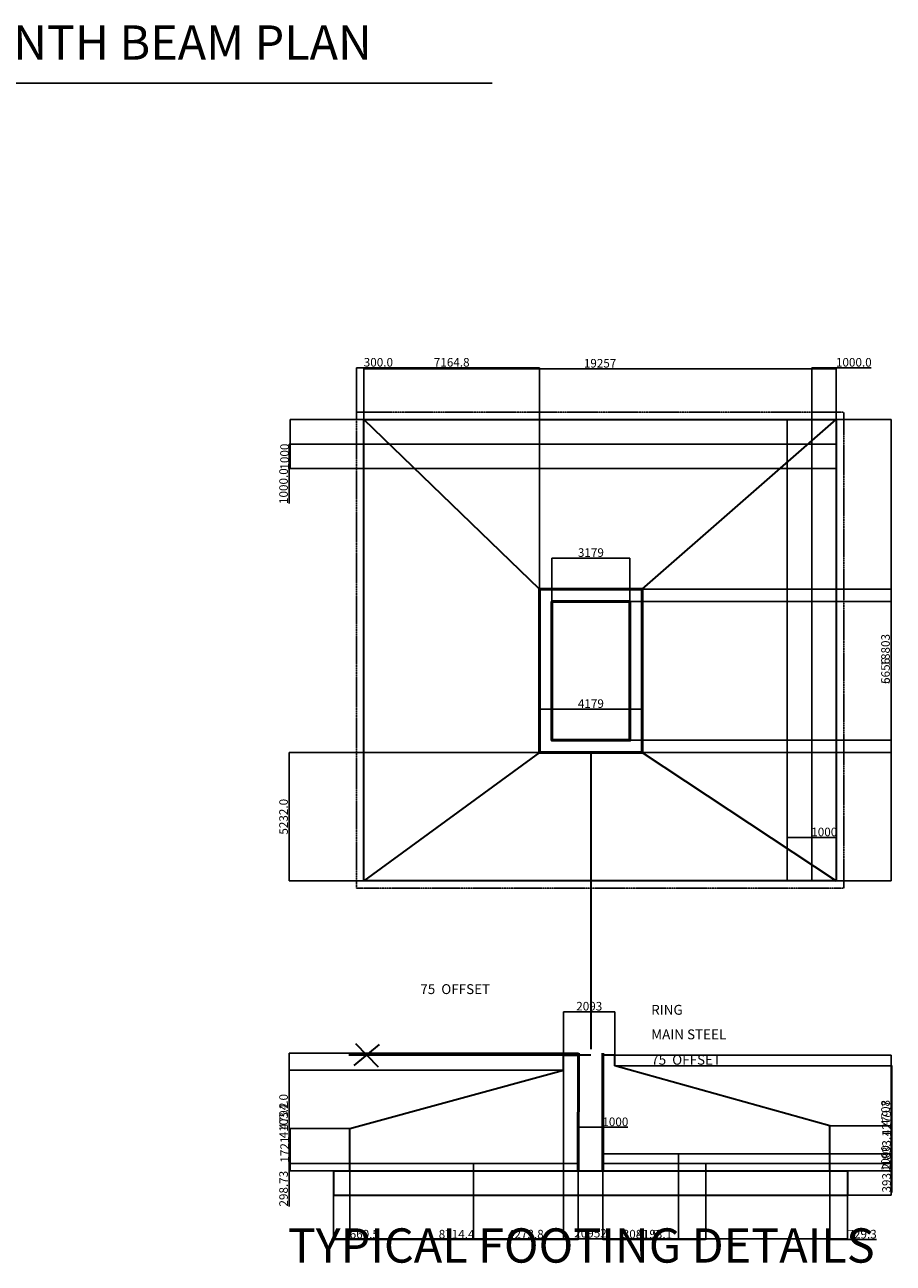
# Model space of a CAD drawing. Units: millimetres. Extents: x -2405 to 73447, y 417 to 55353.
# Tile 3 of 3: x 38054 to 73447, y 4879 to 55353. Entities that reach past the tile are written whole.
import ezdxf

# ---------------------------------------------------------------- set-up
doc = ezdxf.new("R2010")
doc.units = ezdxf.units.MM
doc.linetypes.add('DASHED', pattern=[19.05, 12.7, -6.35])
for name, color, linetype, lineweight in [('S-ANNO-DIMS', 2, 'Continuous', 18), ('S-ANNO-TEXT', 7, 'Continuous', 25), ('S-COLS', 4, 'Continuous', 50), ('S-FNDN', 3, 'Continuous', 35), ('S-FNDN-HIDN', 8, 'DASHED', 25), ('S-REIN', 1, 'Continuous', 25)]:
    doc.layers.add(name, color=color, linetype=linetype, lineweight=lineweight)
doc.styles.get("Standard").update_dxf_attribs({"font": 'arial.ttf'})
doc.dimstyles.new('ISO-25', dxfattribs={"dimtxt": 350, "dimasz": 2.5, "dimexe": 1.25, "dimexo": 0.625, "dimtad": 1, "dimdec": 0, "dimtxsty": 'Standard', "dimcen": 2.5, "dimadec": 0, "dimazin": 0, "dimtfac": 1, "dimtdec": 0, "dimtmove": 0, "dimatfit": 3, "dimfxl": 1, "dimarcsym": 0})

# ---------------------------------------------------------------- blocks, each defined once
blk = doc.blocks.new('*D23')
at = {"layer": 'Defpoints', "color": 0, "transparency": 16777216}
for p in [(71128, 41333), (51872, 39263), (71128, 39263)]:
    blk.add_point(p, dxfattribs=at)
at = {"layer": 'S-ANNO-DIMS', "color": 0, "lineweight": -2, "transparency": 16777216}
for p, q in [((51872, 39263), (51872, 41334)), ((51874, 41333), (71126, 41333)), ((71128, 39263), (71128, 41334))]:
    blk.add_line(p, q, dxfattribs=at)
at = {"layer": 'S-ANNO-DIMS', "color": 0, "transparency": 16777216}
for points in [[(51874, 41333), (51874, 41332), (51872, 41333)], [(71126, 41333), (71126, 41332), (71128, 41333)]]:
    blk.add_solid(points, dxfattribs=at)
at = {"layer": 'S-ANNO-DIMS', "color": 0, "transparency": 16777216, "insert": (61500, 41512), "char_height": 350, "attachment_point": 5}
blk.add_mtext('19257', dxfattribs=at)
blk = doc.blocks.new('*D24')
at = {"layer": 'Defpoints', "color": 0, "transparency": 16777216}
for p in [(71128, 39263), (71128, 20460), (73357, 20460)]:
    blk.add_point(p, dxfattribs=at)
at = {"layer": 'S-ANNO-DIMS', "color": 0, "lineweight": -2, "transparency": 16777216}
for p, q in [((71129, 39263), (73358, 39263)), ((73357, 39260), (73357, 20463)), ((71129, 20460), (73358, 20460))]:
    blk.add_line(p, q, dxfattribs=at)
at = {"layer": 'S-ANNO-DIMS', "color": 0, "transparency": 16777216}
for points in [[(73357, 39260), (73358, 39260), (73357, 39263)], [(73357, 20463), (73358, 20463), (73357, 20460)]]:
    blk.add_solid(points, dxfattribs=at)
at = {"layer": 'S-ANNO-DIMS', "color": 0, "transparency": 16777216, "insert": (73178, 29862), "char_height": 350, "attachment_point": 5, "rotation": 90}
blk.add_mtext('18803', dxfattribs=at)
blk = doc.blocks.new('*D25')
at = {"layer": 'Defpoints', "color": 0, "transparency": 16777216}
for p in [(63215, 27462), (59036, 25692), (63215, 25692)]:
    blk.add_point(p, dxfattribs=at)
at = {"layer": 'S-ANNO-DIMS', "color": 0, "lineweight": -2, "transparency": 16777216}
for p, q in [((59036, 25693), (59036, 27464)), ((59039, 27462), (63213, 27462)), ((63215, 25693), (63215, 27464))]:
    blk.add_line(p, q, dxfattribs=at)
at = {"layer": 'S-ANNO-DIMS', "color": 0, "transparency": 16777216}
for points in [[(59039, 27463), (59039, 27462), (59036, 27462)], [(63213, 27463), (63213, 27462), (63215, 27462)]]:
    blk.add_solid(points, dxfattribs=at)
at = {"layer": 'S-ANNO-DIMS', "color": 0, "transparency": 16777216, "insert": (61126, 27642), "char_height": 350, "attachment_point": 5}
blk.add_mtext('4179', dxfattribs=at)
blk = doc.blocks.new('*D26')
at = {"layer": 'Defpoints', "color": 0, "transparency": 16777216}
for p in [(63215, 32348), (63215, 25692), (73357, 25692)]:
    blk.add_point(p, dxfattribs=at)
at = {"layer": 'S-ANNO-DIMS', "color": 0, "lineweight": -2, "transparency": 16777216}
for p, q in [((63216, 32348), (73358, 32348)), ((73357, 32346), (73357, 25695)), ((63216, 25692), (73358, 25692))]:
    blk.add_line(p, q, dxfattribs=at)
at = {"layer": 'S-ANNO-DIMS', "color": 0, "transparency": 16777216}
for points in [[(73357, 32346), (73358, 32346), (73357, 32348)], [(73357, 25695), (73358, 25695), (73357, 25692)]]:
    blk.add_solid(points, dxfattribs=at)
at = {"layer": 'S-ANNO-DIMS', "color": 0, "transparency": 16777216, "insert": (73178, 29020), "char_height": 350, "attachment_point": 5, "rotation": 90}
blk.add_mtext('6656', dxfattribs=at)
blk = doc.blocks.new('*D27')
at = {"layer": 'Defpoints', "color": 0, "transparency": 16777216}
for p in [(62715, 33618), (59536, 31848), (62715, 31848)]:
    blk.add_point(p, dxfattribs=at)
at = {"layer": 'S-ANNO-DIMS', "color": 0, "lineweight": -2, "transparency": 16777216}
for p, q in [((59536, 31849), (59536, 33619)), ((59539, 33618), (62713, 33618)), ((62715, 31849), (62715, 33619))]:
    blk.add_line(p, q, dxfattribs=at)
at = {"layer": 'S-ANNO-DIMS', "color": 0, "transparency": 16777216}
for points in [[(59539, 33618), (59539, 33618), (59536, 33618)], [(62713, 33618), (62713, 33618), (62715, 33618)]]:
    blk.add_solid(points, dxfattribs=at)
at = {"layer": 'S-ANNO-DIMS', "color": 0, "transparency": 16777216, "insert": (61126, 33797), "char_height": 350, "attachment_point": 5}
blk.add_mtext('3179', dxfattribs=at)
blk = doc.blocks.new('*D28')
at = {"layer": 'Defpoints', "color": 0, "transparency": 16777216}
for p in [(62715, 31848), (62715, 26192), (73357, 26192)]:
    blk.add_point(p, dxfattribs=at)
at = {"layer": 'S-ANNO-DIMS', "color": 0, "lineweight": -2, "transparency": 16777216}
for p, q in [((62716, 31848), (73358, 31848)), ((73357, 31846), (73357, 26195)), ((62716, 26192), (73358, 26192))]:
    blk.add_line(p, q, dxfattribs=at)
at = {"layer": 'S-ANNO-DIMS', "color": 0, "transparency": 16777216}
for points in [[(73357, 31846), (73358, 31846), (73357, 31848)], [(73357, 26195), (73358, 26195), (73357, 26192)]]:
    blk.add_solid(points, dxfattribs=at)
at = {"layer": 'S-ANNO-DIMS', "color": 0, "transparency": 16777216, "insert": (73178, 29020), "char_height": 350, "attachment_point": 5, "rotation": 90}
blk.add_mtext('5656', dxfattribs=at)
blk = doc.blocks.new('*D29')
at = {"layer": 'Defpoints', "color": 0, "transparency": 16777216}
for p in [(70128, 22230), (69128, 20460), (70128, 20460)]:
    blk.add_point(p, dxfattribs=at)
at = {"layer": 'S-ANNO-DIMS', "color": 0, "lineweight": -2, "transparency": 16777216}
for p, q in [((69128, 20461), (69128, 22232)), ((69131, 22230), (70126, 22230)), ((70128, 20461), (70128, 22232)), ((70128, 22230), (71143, 22230))]:
    blk.add_line(p, q, dxfattribs=at)
at = {"layer": 'S-ANNO-DIMS', "color": 0, "transparency": 16777216}
for points in [[(69131, 22231), (69131, 22230), (69128, 22230)], [(70126, 22231), (70126, 22230), (70128, 22230)]]:
    blk.add_solid(points, dxfattribs=at)
at = {"layer": 'S-ANNO-DIMS', "color": 0, "transparency": 16777216, "insert": (70637, 22410), "char_height": 350, "attachment_point": 5}
blk.add_mtext('1000', dxfattribs=at)
blk = doc.blocks.new('*D30')
at = {"layer": 'Defpoints', "color": 0, "transparency": 16777216}
for p in [(51872, 39263), (48866, 38263), (51872, 38263)]:
    blk.add_point(p, dxfattribs=at)
at = {"layer": 'S-ANNO-DIMS', "color": 0, "lineweight": -2, "transparency": 16777216}
for p, q in [((51871, 39263), (48864, 39263)), ((48866, 39260), (48866, 38265)), ((51871, 38263), (48864, 38263)), ((48866, 38263), (48866, 37248))]:
    blk.add_line(p, q, dxfattribs=at)
at = {"layer": 'S-ANNO-DIMS', "color": 0, "transparency": 16777216}
for points in [[(48865, 39260), (48866, 39260), (48866, 39263)], [(48865, 38265), (48866, 38265), (48866, 38263)]]:
    blk.add_solid(points, dxfattribs=at)
at = {"layer": 'S-ANNO-DIMS', "color": 0, "transparency": 16777216, "insert": (48686, 37754), "char_height": 350, "attachment_point": 5, "rotation": 90}
blk.add_mtext('1000', dxfattribs=at)
blk = doc.blocks.new('*D31')
at = {"layer": 'Defpoints', "color": 0, "transparency": 16777216}
for p in [(50636, 7650), (71587, 7650), (71587, 5880)]:
    blk.add_point(p, dxfattribs=at)
at = {"layer": 'S-ANNO-DIMS', "color": 0, "lineweight": -2, "transparency": 16777216}
for p, q in [((50636, 7650), (50636, 5879)), ((71587, 7650), (71587, 5879)), ((50638, 5880), (71585, 5880))]:
    blk.add_line(p, q, dxfattribs=at)
at = {"layer": 'S-ANNO-DIMS', "color": 0, "transparency": 16777216}
for points in [[(50638, 5881), (50638, 5880), (50636, 5880)], [(71585, 5881), (71585, 5880), (71587, 5880)]]:
    blk.add_solid(points, dxfattribs=at)
at = {"layer": 'S-ANNO-DIMS', "color": 0, "transparency": 16777216, "insert": (61111, 6059), "char_height": 350, "attachment_point": 5}
blk.add_mtext('20952', dxfattribs=at)
blk = doc.blocks.new('*D32')
at = {"layer": 'Defpoints', "color": 0, "transparency": 16777216}
for p in [(71587, 8650), (73357, 8650), (71587, 7650)]:
    blk.add_point(p, dxfattribs=at)
at = {"layer": 'S-ANNO-DIMS', "color": 0, "lineweight": -2, "transparency": 16777216}
for p, q in [((73357, 8650), (73357, 9665)), ((71588, 8650), (73358, 8650)), ((73357, 7653), (73357, 8648)), ((71588, 7650), (73358, 7650))]:
    blk.add_line(p, q, dxfattribs=at)
at = {"layer": 'S-ANNO-DIMS', "color": 0, "transparency": 16777216}
for points in [[(73357, 8648), (73358, 8648), (73357, 8650)], [(73357, 7653), (73358, 7653), (73357, 7650)]]:
    blk.add_solid(points, dxfattribs=at)
at = {"layer": 'S-ANNO-DIMS', "color": 0, "transparency": 16777216, "insert": (73178, 9159), "char_height": 350, "attachment_point": 5, "rotation": 90}
blk.add_mtext('1000', dxfattribs=at)
blk = doc.blocks.new('*D33')
at = {"layer": 'Defpoints', "color": 0, "transparency": 16777216}
for p in [(48866, 10371), (51296, 10371), (51296, 8650)]:
    blk.add_point(p, dxfattribs=at)
at = {"layer": 'S-ANNO-DIMS', "color": 0, "lineweight": -2, "transparency": 16777216}
for p, q in [((51295, 10371), (48864, 10371)), ((48866, 8653), (48866, 10369)), ((51295, 8650), (48864, 8650))]:
    blk.add_line(p, q, dxfattribs=at)
at = {"layer": 'S-ANNO-DIMS', "color": 0, "transparency": 16777216}
for points in [[(48865, 10369), (48866, 10369), (48866, 10371)], [(48865, 8653), (48866, 8653), (48866, 8650)]]:
    blk.add_solid(points, dxfattribs=at)
at = {"layer": 'S-ANNO-DIMS', "color": 0, "transparency": 16777216, "insert": (48689, 9511), "char_height": 350, "attachment_point": 5, "rotation": 90}
blk.add_mtext('1721', dxfattribs=at)
blk = doc.blocks.new('*D34')
at = {"layer": 'Defpoints', "color": 0, "transparency": 16777216}
for p in [(62103, 13359), (70858, 8650), (73357, 8650)]:
    blk.add_point(p, dxfattribs=at)
at = {"layer": 'S-ANNO-DIMS', "color": 0, "lineweight": -2, "transparency": 16777216}
for p, q in [((62104, 13359), (73358, 13359)), ((73357, 13356), (73357, 8653)), ((70858, 8650), (73358, 8650))]:
    blk.add_line(p, q, dxfattribs=at)
at = {"layer": 'S-ANNO-DIMS', "color": 0, "transparency": 16777216}
for points in [[(73357, 13356), (73358, 13356), (73357, 13359)], [(73357, 8653), (73358, 8653), (73357, 8650)]]:
    blk.add_solid(points, dxfattribs=at)
at = {"layer": 'S-ANNO-DIMS', "color": 0, "transparency": 16777216, "insert": (73178, 11004), "char_height": 350, "attachment_point": 5, "rotation": 90}
blk.add_mtext('4708', dxfattribs=at)
blk = doc.blocks.new('*D35')
at = {"layer": 'Defpoints', "color": 0, "transparency": 16777216}
for p in [(62105, 15129), (60011, 13361), (62103, 13359)]:
    blk.add_point(p, dxfattribs=at)
at = {"layer": 'S-ANNO-DIMS', "color": 0, "lineweight": -2, "transparency": 16777216}
for p, q in [((60011, 13361), (60012, 15132)), ((60015, 15131), (62103, 15129)), ((62103, 13359), (62105, 15130))]:
    blk.add_line(p, q, dxfattribs=at)
at = {"layer": 'S-ANNO-DIMS', "color": 0, "transparency": 16777216}
for points in [[(60015, 15131), (60015, 15130), (60012, 15131)], [(62103, 15129), (62103, 15128), (62105, 15129)]]:
    blk.add_solid(points, dxfattribs=at)
at = {"layer": 'S-ANNO-DIMS', "color": 0, "transparency": 16777216, "insert": (61059, 15309), "char_height": 350, "attachment_point": 5, "rotation": 359.9376}
blk.add_mtext('2093', dxfattribs=at)
blk = doc.blocks.new('*D36')
at = {"layer": 'Defpoints', "color": 0, "transparency": 16777216}
for p in [(61613, 10420), (60611, 8651), (61611, 8650)]:
    blk.add_point(p, dxfattribs=at)
at = {"layer": 'S-ANNO-DIMS', "color": 0, "lineweight": -2, "transparency": 16777216}
for p, q in [((60611, 8651), (60613, 10422)), ((60616, 10421), (61611, 10420)), ((61611, 8650), (61613, 10421)), ((61613, 10420), (62628, 10418))]:
    blk.add_line(p, q, dxfattribs=at)
at = {"layer": 'S-ANNO-DIMS', "color": 0, "transparency": 16777216}
for points in [[(60616, 10421), (60616, 10420), (60613, 10421)], [(61611, 10420), (61611, 10419), (61613, 10420)]]:
    blk.add_solid(points, dxfattribs=at)
at = {"layer": 'S-ANNO-DIMS', "color": 0, "transparency": 16777216, "insert": (62122, 10598), "char_height": 350, "attachment_point": 5, "rotation": 359.9376}
blk.add_mtext('1000', dxfattribs=at)
blk = doc.blocks.new('*D46')
at = {"layer": 'Defpoints', "color": 0, "transparency": 16777216}
for p in [(59036, 41373), (51872, 39263), (59036, 32348)]:
    blk.add_point(p, dxfattribs=at)
at = {"layer": 'S-ANNO-DIMS', "color": 0, "lineweight": -2, "transparency": 16777216}
for p, q in [((51872, 39263), (51872, 41374)), ((51874, 41373), (59034, 41373)), ((59036, 32349), (59036, 41374))]:
    blk.add_line(p, q, dxfattribs=at)
at = {"layer": 'S-ANNO-DIMS', "color": 0, "transparency": 16777216}
for points in [[(51874, 41373), (51874, 41372), (51872, 41373)], [(59034, 41373), (59034, 41372), (59036, 41373)]]:
    blk.add_solid(points, dxfattribs=at)
at = {"layer": 'S-ANNO-DIMS', "color": 0, "transparency": 16777216, "insert": (55454, 41552), "char_height": 350, "attachment_point": 5}
blk.add_mtext('7164.8', dxfattribs=at)
blk = doc.blocks.new('*D47')
at = {"layer": 'Defpoints', "color": 0, "transparency": 16777216}
for p in [(59036, 25692), (48826, 20460), (51872, 20460)]:
    blk.add_point(p, dxfattribs=at)
at = {"layer": 'S-ANNO-DIMS', "color": 0, "lineweight": -2, "transparency": 16777216}
for p, q in [((59036, 25692), (48824, 25692)), ((48826, 25690), (48826, 20463)), ((51871, 20460), (48824, 20460))]:
    blk.add_line(p, q, dxfattribs=at)
at = {"layer": 'S-ANNO-DIMS', "color": 0, "transparency": 16777216}
for points in [[(48825, 25690), (48826, 25690), (48826, 25692)], [(48825, 20463), (48826, 20463), (48826, 20460)]]:
    blk.add_solid(points, dxfattribs=at)
at = {"layer": 'S-ANNO-DIMS', "color": 0, "transparency": 16777216, "insert": (48646, 23076), "char_height": 350, "attachment_point": 5, "rotation": 90}
blk.add_mtext('5232.0', dxfattribs=at)
blk = doc.blocks.new('*D48')
at = {"layer": 'Defpoints', "color": 0, "transparency": 16777216}
for p in [(51872, 38263), (48826, 37263), (51872, 37263)]:
    blk.add_point(p, dxfattribs=at)
at = {"layer": 'S-ANNO-DIMS', "color": 0, "lineweight": -2, "transparency": 16777216}
for p, q in [((51871, 38263), (48824, 38263)), ((48826, 38260), (48826, 37265)), ((51871, 37263), (48824, 37263)), ((48826, 37263), (48826, 35840))]:
    blk.add_line(p, q, dxfattribs=at)
at = {"layer": 'S-ANNO-DIMS', "color": 0, "transparency": 16777216}
for points in [[(48825, 38260), (48826, 38260), (48826, 38263)], [(48825, 37265), (48826, 37265), (48826, 37263)]]:
    blk.add_solid(points, dxfattribs=at)
at = {"layer": 'S-ANNO-DIMS', "color": 0, "transparency": 16777216, "insert": (48646, 36550), "char_height": 350, "attachment_point": 5, "rotation": 90}
blk.add_mtext('1000.0', dxfattribs=at)
blk = doc.blocks.new('*D49')
at = {"layer": 'Defpoints', "color": 0, "transparency": 16777216}
for p in [(71128, 41373), (70128, 39263), (71128, 39263)]:
    blk.add_point(p, dxfattribs=at)
at = {"layer": 'S-ANNO-DIMS', "color": 0, "lineweight": -2, "transparency": 16777216}
for p, q in [((70128, 39263), (70128, 41374)), ((70131, 41373), (71126, 41373)), ((71128, 39263), (71128, 41374)), ((71128, 41373), (72551, 41373))]:
    blk.add_line(p, q, dxfattribs=at)
at = {"layer": 'S-ANNO-DIMS', "color": 0, "transparency": 16777216}
for points in [[(70131, 41373), (70131, 41372), (70128, 41373)], [(71126, 41373), (71126, 41372), (71128, 41373)]]:
    blk.add_solid(points, dxfattribs=at)
at = {"layer": 'S-ANNO-DIMS', "color": 0, "transparency": 16777216, "insert": (71841, 41552), "char_height": 350, "attachment_point": 5}
blk.add_mtext('1000.0', dxfattribs=at)
blk = doc.blocks.new('*D50')
at = {"layer": 'Defpoints', "color": 0, "transparency": 16777216}
for p in [(51872, 41373), (51572, 39563), (51872, 39263)]:
    blk.add_point(p, dxfattribs=at)
at = {"layer": 'S-ANNO-DIMS', "color": 0, "lineweight": -2, "transparency": 16777216}
for p, q in [((51572, 39563), (51572, 41374)), ((51574, 41373), (51869, 41373)), ((51872, 39263), (51872, 41374)), ((51872, 41373), (53055, 41373))]:
    blk.add_line(p, q, dxfattribs=at)
at = {"layer": 'S-ANNO-DIMS', "color": 0, "transparency": 16777216}
for points in [[(51574, 41373), (51574, 41372), (51572, 41373)], [(51869, 41373), (51869, 41372), (51872, 41373)]]:
    blk.add_solid(points, dxfattribs=at)
at = {"layer": 'S-ANNO-DIMS', "color": 0, "transparency": 16777216, "insert": (52465, 41552), "char_height": 350, "attachment_point": 5}
blk.add_mtext('300.0', dxfattribs=at)
blk = doc.blocks.new('*D51')
at = {"layer": 'Defpoints', "color": 0, "transparency": 16777216}
for p in [(50636, 8650), (51296, 8650), (51296, 5840)]:
    blk.add_point(p, dxfattribs=at)
at = {"layer": 'S-ANNO-DIMS', "color": 0, "lineweight": -2, "transparency": 16777216}
for p, q in [((50636, 8650), (50636, 5839)), ((51296, 8650), (51296, 5839)), ((50638, 5840), (51294, 5840)), ((51296, 5840), (52485, 5840))]:
    blk.add_line(p, q, dxfattribs=at)
at = {"layer": 'S-ANNO-DIMS', "color": 0, "transparency": 16777216}
for points in [[(50638, 5841), (50638, 5840), (50636, 5840)], [(51294, 5841), (51294, 5840), (51296, 5840)]]:
    blk.add_solid(points, dxfattribs=at)
at = {"layer": 'S-ANNO-DIMS', "color": 0, "transparency": 16777216, "insert": (51892, 6019), "char_height": 350, "attachment_point": 5}
blk.add_mtext('660.5', dxfattribs=at)
blk = doc.blocks.new('*D52')
at = {"layer": 'Defpoints', "color": 0, "transparency": 16777216}
for p in [(70858, 8650), (71587, 8650), (71587, 5840)]:
    blk.add_point(p, dxfattribs=at)
at = {"layer": 'S-ANNO-DIMS', "color": 0, "lineweight": -2, "transparency": 16777216}
for p, q in [((70858, 8650), (70858, 5839)), ((71587, 8650), (71587, 5839)), ((70860, 5840), (71585, 5840)), ((71587, 5840), (72769, 5840))]:
    blk.add_line(p, q, dxfattribs=at)
at = {"layer": 'S-ANNO-DIMS', "color": 0, "transparency": 16777216}
for points in [[(70860, 5841), (70860, 5840), (70858, 5840)], [(71585, 5841), (71585, 5840), (71587, 5840)]]:
    blk.add_solid(points, dxfattribs=at)
at = {"layer": 'S-ANNO-DIMS', "color": 0, "transparency": 16777216, "insert": (72179, 6020), "char_height": 350, "attachment_point": 5}
blk.add_mtext('729.3', dxfattribs=at)
blk = doc.blocks.new('*D53')
at = {"layer": 'Defpoints', "color": 0, "transparency": 16777216}
for p in [(70858, 10483), (70858, 8650), (73397, 8650)]:
    blk.add_point(p, dxfattribs=at)
at = {"layer": 'S-ANNO-DIMS', "color": 0, "lineweight": -2, "transparency": 16777216}
for p, q in [((70858, 10483), (73398, 10483)), ((73397, 10481), (73397, 8653)), ((70858, 8650), (73398, 8650))]:
    blk.add_line(p, q, dxfattribs=at)
at = {"layer": 'S-ANNO-DIMS', "color": 0, "transparency": 16777216}
for points in [[(73397, 10481), (73398, 10481), (73397, 10483)], [(73397, 8653), (73398, 8653), (73397, 8650)]]:
    blk.add_solid(points, dxfattribs=at)
at = {"layer": 'S-ANNO-DIMS', "color": 0, "transparency": 16777216, "insert": (73218, 9567), "char_height": 350, "attachment_point": 5, "rotation": 90}
blk.add_mtext('1833.1', dxfattribs=at)
blk = doc.blocks.new('*D54')
at = {"layer": 'Defpoints', "color": 0, "transparency": 16777216}
for p in [(60011, 12754), (48826, 8651), (60611, 8651)]:
    blk.add_point(p, dxfattribs=at)
at = {"layer": 'S-ANNO-DIMS', "color": 0, "lineweight": -2, "transparency": 16777216}
for p, q in [((60010, 12754), (48824, 12754)), ((48826, 12751), (48826, 8653)), ((60611, 8651), (48824, 8651))]:
    blk.add_line(p, q, dxfattribs=at)
at = {"layer": 'S-ANNO-DIMS', "color": 0, "transparency": 16777216}
for points in [[(48825, 12751), (48826, 12751), (48826, 12754)], [(48825, 8653), (48826, 8653), (48826, 8651)]]:
    blk.add_solid(points, dxfattribs=at)
at = {"layer": 'S-ANNO-DIMS', "color": 0, "transparency": 16777216, "insert": (48646, 10702), "char_height": 350, "attachment_point": 5, "rotation": 90}
blk.add_mtext('4103.2', dxfattribs=at)
blk = doc.blocks.new('*D55')
at = {"layer": 'Defpoints', "color": 0, "transparency": 16777216}
for p in [(60011, 12754), (51296, 10371), (60011, 5840)]:
    blk.add_point(p, dxfattribs=at)
at = {"layer": 'S-ANNO-DIMS', "color": 0, "lineweight": -2, "transparency": 16777216}
for p, q in [((60011, 12753), (60011, 5839)), ((51296, 10370), (51296, 5839)), ((51299, 5840), (60008, 5840))]:
    blk.add_line(p, q, dxfattribs=at)
at = {"layer": 'S-ANNO-DIMS', "color": 0, "transparency": 16777216}
for points in [[(51299, 5841), (51299, 5840), (51296, 5840)], [(60008, 5841), (60008, 5840), (60011, 5840)]]:
    blk.add_solid(points, dxfattribs=at)
at = {"layer": 'S-ANNO-DIMS', "color": 0, "transparency": 16777216, "insert": (55653, 6019), "char_height": 350, "attachment_point": 5}
blk.add_mtext('8714.4', dxfattribs=at)
blk = doc.blocks.new('*D56')
at = {"layer": 'Defpoints', "color": 0, "transparency": 16777216}
for p in [(62103, 12929), (61611, 8650), (73397, 8650)]:
    blk.add_point(p, dxfattribs=at)
at = {"layer": 'S-ANNO-DIMS', "color": 0, "lineweight": -2, "transparency": 16777216}
for p, q in [((62104, 12929), (73398, 12929)), ((73397, 12927), (73397, 8652)), ((61612, 8650), (73398, 8650))]:
    blk.add_line(p, q, dxfattribs=at)
at = {"layer": 'S-ANNO-DIMS', "color": 0, "transparency": 16777216}
for points in [[(73397, 12927), (73398, 12927), (73397, 12929)], [(73397, 8652), (73398, 8652), (73397, 8650)]]:
    blk.add_solid(points, dxfattribs=at)
at = {"layer": 'S-ANNO-DIMS', "color": 0, "transparency": 16777216, "insert": (73218, 10789), "char_height": 350, "attachment_point": 5, "rotation": 90}
blk.add_mtext('4279.7', dxfattribs=at)
blk = doc.blocks.new('*D57')
at = {"layer": 'Defpoints', "color": 0, "transparency": 16777216}
for p in [(56338, 8949), (60612, 8949), (60612, 5840)]:
    blk.add_point(p, dxfattribs=at)
at = {"layer": 'S-ANNO-DIMS', "color": 0, "lineweight": -2, "transparency": 16777216}
for p, q in [((56338, 8948), (56338, 5839)), ((60612, 8948), (60612, 5839)), ((56340, 5840), (60609, 5840))]:
    blk.add_line(p, q, dxfattribs=at)
at = {"layer": 'S-ANNO-DIMS', "color": 0, "transparency": 16777216}
for points in [[(56340, 5841), (56340, 5840), (56338, 5840)], [(60609, 5841), (60609, 5840), (60612, 5840)]]:
    blk.add_solid(points, dxfattribs=at)
at = {"layer": 'S-ANNO-DIMS', "color": 0, "transparency": 16777216, "insert": (58475, 6020), "char_height": 350, "attachment_point": 5}
blk.add_mtext('4273.8', dxfattribs=at)
blk = doc.blocks.new('*D58')
at = {"layer": 'Defpoints', "color": 0, "transparency": 16777216}
for p in [(48826, 8650), (56338, 8949), (56338, 8650)]:
    blk.add_point(p, dxfattribs=at)
at = {"layer": 'S-ANNO-DIMS', "color": 0, "lineweight": -2, "transparency": 16777216}
for p, q in [((56337, 8949), (48824, 8949)), ((56337, 8650), (48824, 8650)), ((48826, 8946), (48826, 8653)), ((48826, 8650), (48826, 7187))]:
    blk.add_line(p, q, dxfattribs=at)
at = {"layer": 'S-ANNO-DIMS', "color": 0, "transparency": 16777216}
for points in [[(48825, 8946), (48826, 8946), (48826, 8949)], [(48825, 8653), (48826, 8653), (48826, 8650)]]:
    blk.add_solid(points, dxfattribs=at)
at = {"layer": 'S-ANNO-DIMS', "color": 0, "transparency": 16777216, "insert": (48646, 7918), "char_height": 350, "attachment_point": 5, "rotation": 90}
blk.add_mtext('298.73', dxfattribs=at)
blk = doc.blocks.new('*D59')
at = {"layer": 'Defpoints', "color": 0, "transparency": 16777216}
for p in [(61612, 8949), (65805, 8949), (65805, 5840)]:
    blk.add_point(p, dxfattribs=at)
at = {"layer": 'S-ANNO-DIMS', "color": 0, "lineweight": -2, "transparency": 16777216}
for p, q in [((61612, 8948), (61612, 5839)), ((65805, 8948), (65805, 5839)), ((61614, 5840), (65802, 5840))]:
    blk.add_line(p, q, dxfattribs=at)
at = {"layer": 'S-ANNO-DIMS', "color": 0, "transparency": 16777216}
for points in [[(61614, 5841), (61614, 5840), (61612, 5840)], [(65802, 5841), (65802, 5840), (65805, 5840)]]:
    blk.add_solid(points, dxfattribs=at)
at = {"layer": 'S-ANNO-DIMS', "color": 0, "transparency": 16777216, "insert": (63708, 6020), "char_height": 350, "attachment_point": 5}
blk.add_mtext('4193.1', dxfattribs=at)
blk = doc.blocks.new('*D60')
at = {"layer": 'Defpoints', "color": 0, "transparency": 16777216}
for p in [(61612, 9342), (64694, 9342), (64694, 5840)]:
    blk.add_point(p, dxfattribs=at)
at = {"layer": 'S-ANNO-DIMS', "color": 0, "lineweight": -2, "transparency": 16777216}
for p, q in [((61612, 9341), (61612, 5839)), ((64694, 9341), (64694, 5839)), ((61615, 5840), (64691, 5840))]:
    blk.add_line(p, q, dxfattribs=at)
at = {"layer": 'S-ANNO-DIMS', "color": 0, "transparency": 16777216}
for points in [[(61615, 5841), (61615, 5840), (61612, 5840)], [(64691, 5841), (64691, 5840), (64694, 5840)]]:
    blk.add_solid(points, dxfattribs=at)
at = {"layer": 'S-ANNO-DIMS', "color": 0, "transparency": 16777216, "insert": (63153, 6020), "char_height": 350, "attachment_point": 5}
blk.add_mtext('3081.5', dxfattribs=at)
blk = doc.blocks.new('*D61')
at = {"layer": 'Defpoints', "color": 0, "transparency": 16777216}
for p in [(64694, 9342), (64694, 8949), (73397, 8949)]:
    blk.add_point(p, dxfattribs=at)
at = {"layer": 'S-ANNO-DIMS', "color": 0, "lineweight": -2, "transparency": 16777216}
for p, q in [((64694, 9342), (73398, 9342)), ((73397, 9340), (73397, 8951)), ((64694, 8949), (73398, 8949)), ((73397, 8949), (73397, 7768))]:
    blk.add_line(p, q, dxfattribs=at)
at = {"layer": 'S-ANNO-DIMS', "color": 0, "transparency": 16777216}
for points in [[(73397, 9340), (73398, 9340), (73397, 9342)], [(73397, 8951), (73398, 8951), (73397, 8949)]]:
    blk.add_solid(points, dxfattribs=at)
at = {"layer": 'S-ANNO-DIMS', "color": 0, "transparency": 16777216, "insert": (73218, 8357), "char_height": 350, "attachment_point": 5, "rotation": 90}
blk.add_mtext('393.2', dxfattribs=at)
blk = doc.blocks.new('*D62')
at = {"layer": 'Defpoints', "color": 0, "transparency": 16777216}
for p in [(60617, 13445), (48826, 8651), (60611, 8651)]:
    blk.add_point(p, dxfattribs=at)
at = {"layer": 'S-ANNO-DIMS', "color": 0, "lineweight": -2, "transparency": 16777216}
for p, q in [((60616, 13445), (48824, 13445)), ((48826, 13442), (48826, 8653)), ((60611, 8651), (48824, 8651))]:
    blk.add_line(p, q, dxfattribs=at)
at = {"layer": 'S-ANNO-DIMS', "color": 0, "transparency": 16777216}
for points in [[(48825, 13442), (48826, 13442), (48826, 13445)], [(48825, 8653), (48826, 8653), (48826, 8651)]]:
    blk.add_solid(points, dxfattribs=at)
at = {"layer": 'S-ANNO-DIMS', "color": 0, "transparency": 16777216, "insert": (48646, 11048), "char_height": 350, "attachment_point": 5, "rotation": 90}
blk.add_mtext('4794.0', dxfattribs=at)

msp = doc.modelspace()

# ---------------------------------------------------------------- linework, layer by layer
at = {"layer": 'S-ANNO-TEXT'}
msp.add_line((-2404.637, 52969.195), (57098.008, 52969.195), dxfattribs=at)
at = {"layer": 'S-COLS'}
for p, q in [((60616.568, 13444.714), (60611.346, 8650.682)), ((61616.567, 13443.625), (61611.346, 8649.593))]:
    msp.add_line(p, q, dxfattribs=at)
for points in [[(59036.384, 32348.004), (63215.45, 32348.004), (63215.45, 25692.289), (59036.384, 25692.289)], [(59536.384, 31848.004), (62715.45, 31848.004), (62715.45, 26192.289), (59536.384, 26192.289)]]:
    msp.add_lwpolyline(points, close=True, dxfattribs=at)
at = {"layer": 'S-FNDN'}
for p, q in [((51871.574, 39262.806), (71128.374, 39262.806)), ((51871.574, 20460.3), (51871.574, 39262.806)), ((59036.384, 32348.004), (51871.574, 39262.806)), ((63215.45, 32348.004), (71128.374, 39262.806)), ((71128.374, 39262.806), (71128.374, 20460.3)), ((59036.384, 25692.289), (51871.574, 20460.3)), ((61125.917, 25692.289), (61125.917, 13608.951)), ((63215.45, 25692.289), (71128.374, 20460.3)), ((71128.374, 20460.3), (51871.574, 20460.3)), ((51479.692, 12939.469), (52507.49, 13796.926)), ((51528.059, 13839.195), (52459.123, 12879.085)), ((61125.917, 13359.612), (51264.684, 13359.612)), ((60010.529, 13360.827), (60616.476, 13360.167)), ((60010.529, 12753.871), (60010.529, 13360.827)), ((62103.494, 13358.547), (61616.475, 13359.078)), ((62103.494, 12929.297), (62103.494, 13358.547)), ((51296.106, 10371.099), (60010.529, 12753.871)), ((70857.857, 10483.211), (62103.494, 12929.297)), ((51296.106, 8650.138), (51296.106, 10371.099)), ((70857.857, 8650.138), (70857.857, 10483.211)), ((50635.56, 8650.138), (71587.132, 8650.138)), ((50635.56, 8650.138), (50635.56, 7650.138)), ((71587.132, 8650.138), (71587.132, 7650.138)), ((50635.56, 7650.138), (71587.132, 7650.138))]:
    msp.add_line(p, q, dxfattribs=at)
at = {"layer": 'S-FNDN-HIDN'}
for p, q in [((51571.574, 39262.806), (51571.574, 39562.806)), ((51571.574, 39562.806), (51871.574, 39562.806)), ((51871.574, 39562.806), (71128.374, 39562.806)), ((71128.374, 39562.806), (71428.374, 39562.806)), ((71428.374, 39562.806), (71428.374, 39262.806)), ((51571.574, 20460.3), (51571.574, 39262.806)), ((71428.374, 39262.806), (71428.374, 20460.3)), ((51571.574, 20460.3), (51571.574, 20160.3)), ((71428.374, 20160.3), (71428.374, 20460.3)), ((51571.574, 20160.3), (51965.914, 20160.3)), ((71128.374, 20160.3), (51871.574, 20160.3)), ((71128.374, 20160.3), (71428.374, 20160.3))]:
    msp.add_line(p, q, dxfattribs=at)
at = {"layer": 'S-REIN'}
for p, q in [((69128.374, 39262.806), (69128.374, 20460.3)), ((70128.374, 39262.806), (70128.374, 20460.3)), ((51871.574, 38262.806), (71128.374, 38262.806)), ((51871.574, 37262.806), (71128.374, 37262.806)), ((61612.1, 9342.045), (64693.588, 9342.045)), ((64693.588, 9342.045), (64693.588, 8948.871)), ((60611.671, 8948.871), (56337.894, 8948.871)), ((56337.894, 8948.871), (56337.894, 8650.138)), ((61611.672, 8948.871), (65804.723, 8948.871)), ((65804.723, 8948.871), (65804.723, 8650.138))]:
    msp.add_line(p, q, dxfattribs=at)

# ---------------------------------------------------------------- texts
at = {"layer": 'S-ANNO-TEXT'}
for s, height, p in [('FOOTING DETAILS COLUMN DETAILS AND PLINTH BEAM PLAN', 1397.07747, (-2368.288, 53931.557)), ('75  OFFSET', 401.9761, (54174.436, 15850.2)), ('RING', 401.9761, (63585.02, 15006.898)), ('MAIN STEEL', 401.9761, (63585.02, 14005.772)), ('75  OFFSET', 401.9761, (63585.02, 12969.861)), ('TYPICAL FOOTING DETAILS', 1397.07747, (48772.972, 4904.19))]:
    msp.add_text(s, height=height, dxfattribs=at).set_placement(p)

# ---------------------------------------------------------------- dimensions: what is measured, and where the dimension line sits
at = {"layer": 'S-ANNO-DIMS'}
for base, p1, p2, override, picture, middle in [((51871.574, 41372.806), (51571.574, 39562.806), (51871.574, 39262.806), {"dimdec": 1, "dimlfac": 1, "dimrnd": 0, "dimzin": 0, "dimdsep": 46, "dimlunit": 2}, '*D50', (52464.518, 41552.251)), ((59036.384, 41372.806), (51871.574, 39262.806), (59036.384, 32348.004), {"dimdec": 1, "dimlfac": 1, "dimrnd": 0, "dimzin": 0, "dimdsep": 46, "dimlunit": 2}, '*D46', (55453.979, 41552.132)), ((71128.374, 41332.806), (51871.574, 39262.806), (71128.374, 39262.806), {"dimdec": 0, "dimlfac": 1, "dimrnd": 0, "dimzin": 0, "dimdsep": 46, "dimlunit": 2}, '*D23', (61499.974, 41512.132)), ((71128.374, 41372.806), (70128.374, 39262.806), (71128.374, 39262.806), {"dimdec": 1, "dimlfac": 1, "dimrnd": 0, "dimzin": 0, "dimdsep": 46, "dimlunit": 2}, '*D49', (71840.93, 41552.132)), ((62715.45, 33618.004), (59536.384, 31848.004), (62715.45, 31848.004), {"dimdec": 0, "dimlfac": 1, "dimrnd": 0, "dimzin": 0, "dimdsep": 46, "dimlunit": 2}, '*D27', (61125.917, 33797.449)), ((63215.45, 27462.289), (59036.384, 25692.289), (63215.45, 25692.289), {"dimdec": 0, "dimlfac": 1, "dimrnd": 0, "dimzin": 0, "dimdsep": 46, "dimlunit": 2}, '*D25', (61125.917, 27641.615)), ((70128.374, 22230.3), (69128.374, 20460.3), (70128.374, 20460.3), {"dimdec": 0, "dimlfac": 1, "dimrnd": 0, "dimzin": 0, "dimdsep": 46, "dimlunit": 2}, '*D29', (70637.041, 22409.626)), ((60010.529, 5840.138), (51296.106, 10371.099), (60010.529, 12753.871), {"dimdec": 1, "dimlfac": 1, "dimrnd": 0, "dimzin": 0, "dimdsep": 46, "dimlunit": 2}, '*D55', (55653.317, 6019.463)), ((64693.588, 5840.138), (61612.1, 9342.045), (64693.588, 9342.045), {"dimdec": 1, "dimlfac": 1, "dimrnd": 0, "dimzin": 0, "dimdsep": 46, "dimlunit": 2}, '*D60', (63152.844, 6019.583)), ((51296.106, 5840.138), (50635.56, 8650.138), (51296.106, 8650.138), {"dimdec": 1, "dimlfac": 1, "dimrnd": 0, "dimzin": 0, "dimdsep": 46, "dimlunit": 2}, '*D51', (51892.035, 6019.463)), ((60611.671, 5840.138), (56337.894, 8948.871), (60611.671, 8948.871), {"dimdec": 1, "dimlfac": 1, "dimrnd": 0, "dimzin": 0, "dimdsep": 46, "dimlunit": 2}, '*D57', (58474.782, 6019.583)), ((65804.723, 5840.138), (61611.672, 8948.871), (65804.723, 8948.871), {"dimdec": 1, "dimlfac": 1, "dimrnd": 0, "dimzin": 0, "dimdsep": 46, "dimlunit": 2}, '*D59', (63708.197, 6019.583)), ((71587.132, 5840.138), (70857.857, 8650.138), (71587.132, 8650.138), {"dimdec": 1, "dimlfac": 1, "dimrnd": 0, "dimzin": 0, "dimdsep": 46, "dimlunit": 2}, '*D52', (72179.36, 6019.583)), ((71587.132, 5880.138), (50635.56, 7650.138), (71587.132, 7650.138), {"dimdec": 0, "dimlfac": 1, "dimrnd": 0, "dimzin": 0, "dimdsep": 46, "dimlunit": 2}, '*D31', (61111.346, 6059.463))]:
    dim = msp.add_linear_dim(base=base, p1=p1, p2=p2, dimstyle='ISO-25', override=override, dxfattribs=at)
    dim.commit()
    dim.dimension.update_dxf_attribs({"geometry": picture, "text_midpoint": middle})
for base, p1, p2, angle, override, picture, middle in [((48865.56, 38262.806), (51871.574, 39262.806), (51871.574, 38262.806), 90, {"dimdec": 0, "dimlfac": 1, "dimrnd": 0, "dimzin": 0, "dimdsep": 46, "dimlunit": 2}, '*D30', (48686.235, 37754.139)), ((73357.132, 20460.3), (71128.374, 39262.806), (71128.374, 20460.3), 90, {"dimdec": 0, "dimlfac": 1, "dimrnd": 0, "dimzin": 0, "dimdsep": 46, "dimlunit": 2}, '*D24', (73177.687, 29861.553)), ((48825.56, 37262.806), (51871.574, 38262.806), (51871.574, 37262.806), 90, {"dimdec": 1, "dimlfac": 1, "dimrnd": 0, "dimzin": 0, "dimdsep": 46, "dimlunit": 2}, '*D48', (48646.235, 36550.251)), ((73357.132, 25692.289), (63215.45, 32348.004), (63215.45, 25692.289), 90, {"dimdec": 0, "dimlfac": 1, "dimrnd": 0, "dimzin": 0, "dimdsep": 46, "dimlunit": 2}, '*D26', (73177.806, 29020.146)), ((73357.132, 26192.289), (62715.45, 31848.004), (62715.45, 26192.289), 90, {"dimdec": 0, "dimlfac": 1, "dimrnd": 0, "dimzin": 0, "dimdsep": 46, "dimlunit": 2}, '*D28', (73177.806, 29020.146)), ((48825.56, 20460.3), (59036.384, 25692.289), (51871.574, 20460.3), 90, {"dimdec": 1, "dimlfac": 1, "dimrnd": 0, "dimzin": 0, "dimdsep": 46, "dimlunit": 2}, '*D47', (48646.115, 23076.295)), ((62105.422, 15128.546), (60010.529, 13360.827), (62103.494, 13358.547), 359.9375924, {"dimdec": 0, "dimlfac": 1, "dimrnd": 0, "dimzin": 0, "dimdsep": 46, "dimlunit": 2}, '*D35', (61059.135, 15309.131)), ((48825.56, 8650.682), (60616.568, 13444.714), (60611.346, 8650.682), 90, {"dimdec": 1, "dimlfac": 1, "dimrnd": 0, "dimzin": 0, "dimdsep": 46, "dimlunit": 2}, '*D62', (48646.235, 11047.698)), ((73357.132, 8650.138), (62103.494, 13358.547), (70857.857, 8650.138), 90, {"dimdec": 0, "dimlfac": 1, "dimrnd": 0, "dimzin": 0, "dimdsep": 46, "dimlunit": 2}, '*D34', (73177.806, 11004.342)), ((48825.56, 8650.682), (60010.529, 12753.871), (60611.346, 8650.682), 90, {"dimdec": 1, "dimlfac": 1, "dimrnd": 0, "dimzin": 0, "dimdsep": 46, "dimlunit": 2}, '*D54', (48646.115, 10702.277)), ((73397.132, 8649.593), (62103.494, 12929.297), (61611.346, 8649.593), 90, {"dimdec": 1, "dimlfac": 1, "dimrnd": 0, "dimzin": 0, "dimdsep": 46, "dimlunit": 2}, '*D56', (73217.806, 10789.445)), ((61613.274, 10419.592), (60611.346, 8650.682), (61611.346, 8649.593), 359.9375924, {"dimdec": 0, "dimlfac": 1, "dimrnd": 0, "dimzin": 0, "dimdsep": 46, "dimlunit": 2}, '*D36', (62122.136, 10598.363)), ((48865.56, 10371.099), (51296.106, 8650.138), (51296.106, 10371.099), 90, {"dimdec": 0, "dimlfac": 1, "dimrnd": 0, "dimzin": 0, "dimdsep": 46, "dimlunit": 2}, '*D33', (48689.219, 9510.618)), ((73397.132, 8650.138), (70857.857, 10483.211), (70857.857, 8650.138), 90, {"dimdec": 1, "dimlfac": 1, "dimrnd": 0, "dimzin": 0, "dimdsep": 46, "dimlunit": 2}, '*D53', (73217.687, 9566.675)), ((73357.132, 8650.138), (71587.132, 7650.138), (71587.132, 8650.138), 90, {"dimdec": 0, "dimlfac": 1, "dimrnd": 0, "dimzin": 0, "dimdsep": 46, "dimlunit": 2}, '*D32', (73177.806, 9158.805)), ((73397.132, 8948.871), (64693.588, 9342.045), (64693.588, 8948.871), 90, {"dimdec": 1, "dimlfac": 1, "dimrnd": 0, "dimzin": 0, "dimdsep": 46, "dimlunit": 2}, '*D61', (73217.687, 8357.121)), ((48825.56, 8650.138), (56337.894, 8948.871), (56337.894, 8650.138), 90, {"dimdec": 2, "dimlfac": 1, "dimrnd": 0, "dimzin": 0, "dimdsep": 46, "dimlunit": 2}, '*D58', (48646.115, 7917.528))]:
    dim = msp.add_linear_dim(base=base, p1=p1, p2=p2, angle=angle, dimstyle='ISO-25', override=override, dxfattribs=at)
    dim.commit()
    dim.dimension.update_dxf_attribs({"geometry": picture, "text_midpoint": middle})

doc.saveas('drawing.dxf')
